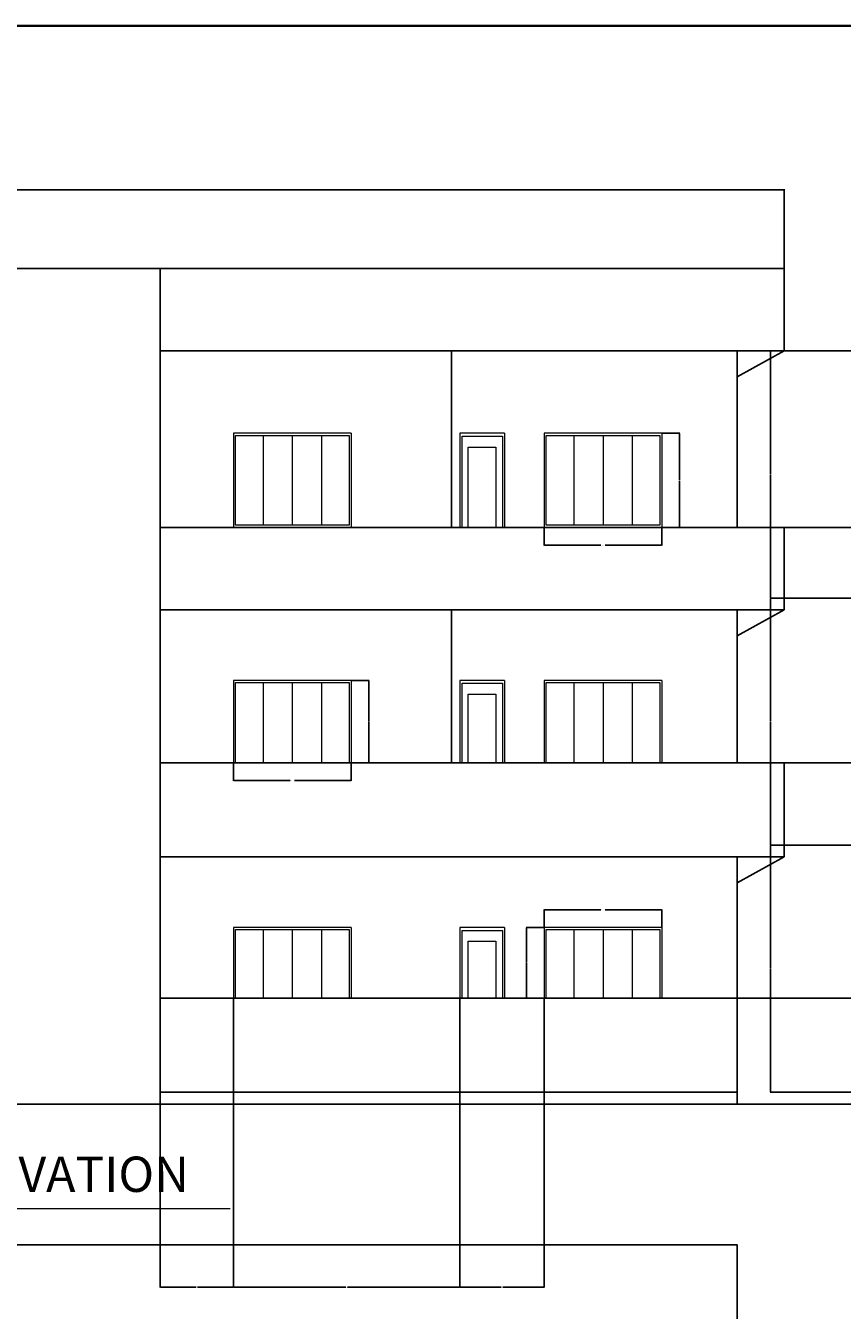
# Model space of a CAD drawing. Units: inches. Extents: x 2120 to 4013, y 1390 to 3019.
# Tile 49 of 59: x 2647 to 3063, y 2364 to 3019. Entities that reach past the tile are written whole.
import ezdxf

# ---------------------------------------------------------------- set-up
doc = ezdxf.new("R2010")
doc.units = ezdxf.units.IN
for name, color, linetype, lineweight in [('A-ANNO-DIMS', 2, 'Continuous', 18), ('A-ANNO-TEXT', 7, 'Continuous', 18), ('A-ANNO-TTLB', 7, 'Continuous', 35), ('A-DOOR', 3, 'Continuous', 18), ('A-ELEV', 7, 'Continuous', 25), ('A-GLAZ', 4, 'Continuous', 18)]:
    doc.layers.add(name, color=color, linetype=linetype, lineweight=lineweight)
doc.styles.get("Standard").update_dxf_attribs({"font": 'arial.ttf'})
doc.dimstyles.get("Standard").update_dxf_attribs({"dimtxt": 0.18, "dimasz": 0.18, "dimexe": 0.18, "dimexo": 0.0625, "dimgap": 0.09, "dimtad": 0, "dimtih": 1, "dimtoh": 1, "dimdec": 4, "dimzin": 0, "dimdsep": 46, "dimtxsty": 'Standard', "dimcen": 0.09, "dimadec": 0, "dimazin": 0, "dimtfac": 1, "dimtdec": 4, "dimtofl": 0, "dimtmove": 0, "dimatfit": 3, "dimfxl": 1, "dimtolj": 1, "dimtzin": 0, "dimarcsym": 0})

# ---------------------------------------------------------------- blocks, each defined once
blk = doc.blocks.new('WIN-ELEV-60IN')
for p, q in [((0, 36), (0, 0)), ((60, 36), (0, 36)), ((0, 36), (0, 0)), ((60, 36), (0, 36)), ((15.15, 34.91), (15.15, 0)), ((30.01, 34.91), (30.01, 0)), ((44.87, 34.91), (44.87, 0)), ((60, 36), (60, 0)), ((60, 36), (60, 0))]:
    blk.add_line(p, q)
blk.add_lwpolyline([(1, 0), (1, 34.91), (59.02, 34.91), (59.02, 0)])
blk = doc.blocks.new('WIN-ELEV-60IN-02')
for p, q in [((0, 42), (0, 0)), ((60, 42), (0, 42)), ((0, 42), (0, 0)), ((60, 42), (0, 42)), ((0, 42), (0, 0)), ((60, 42), (0, 42)), ((15.15, 40.91), (15.15, 0)), ((30.01, 40.91), (30.01, 0)), ((44.87, 40.91), (44.87, 0)), ((60, 42), (60, 0)), ((60, 42), (60, 0)), ((60, 42), (60, 0)), ((0, 36), (0, 0)), ((60, 36), (60, 0))]:
    blk.add_line(p, q)
blk.add_lwpolyline([(1, 0), (1, 40.91), (59.02, 40.91), (59.02, 0)])
blk = doc.blocks.new('WIN-ELEV-60IN-03')
for p, q in [((0, 48), (0, 0)), ((60, 48), (0, 48)), ((0, 48), (0, 0)), ((60, 48), (0, 48)), ((0, 48), (0, 0)), ((60, 48), (0, 48)), ((15.15, 46.91), (15.15, 1.19)), ((30.01, 46.91), (30.01, 1.19)), ((44.87, 46.91), (44.87, 1.19)), ((60, 48), (60, 0)), ((60, 48), (60, 0)), ((60, 48), (60, 0)), ((60, 0), (0, 0)), ((60, 0), (0, 0)), ((60, 0), (0, 0))]:
    blk.add_line(p, q)
blk.add_lwpolyline([(1, 46.91), (59.02, 46.91), (59.02, 1.19), (1, 1.19)], close=True)
blk = doc.blocks.new('*D205')
at = {"layer": 'A-ANNO-DIMS', "color": 0, "lineweight": -2, "transparency": 16777216}
for p, q in [((2911.39, 2559.37), (2911.39, 2568.49)), ((2911.57, 2568.31), (2940.27, 2568.31)), ((2971.21, 2568.31), (2942.51, 2568.31)), ((2971.39, 2559.37), (2971.39, 2568.49))]:
    blk.add_line(p, q, dxfattribs=at)
at = {"layer": 'A-ANNO-DIMS', "color": 0, "transparency": 16777216}
for points in [[(2911.57, 2568.34), (2911.57, 2568.28), (2911.39, 2568.31)], [(2971.21, 2568.34), (2971.21, 2568.28), (2971.39, 2568.31)]]:
    blk.add_solid(points, dxfattribs=at)
at = {"layer": 'Defpoints', "color": 0, "transparency": 16777216}
for p in [(2971.39, 2568.31), (2911.39, 2559.31), (2971.39, 2559.31)]:
    blk.add_point(p, dxfattribs=at)
at = {"layer": 'A-ANNO-DIMS', "color": 0, "transparency": 16777216, "insert": (2941.39, 2568.31), "char_height": 0.18, "attachment_point": 5}
blk.add_mtext('\\A1;WINDOW 60 TYP.', dxfattribs=at)
blk = doc.blocks.new('*D206')
at = {"layer": 'A-ANNO-DIMS', "color": 0, "lineweight": -2, "transparency": 16777216}
for p, q in [((2911.33, 2559.31), (2902.21, 2559.31)), ((2902.39, 2559.13), (2902.39, 2541.49)), ((2902.39, 2523.49), (2902.39, 2541.13)), ((2911.33, 2523.31), (2902.21, 2523.31))]:
    blk.add_line(p, q, dxfattribs=at)
at = {"layer": 'A-ANNO-DIMS', "color": 0, "transparency": 16777216}
for points in [[(2902.36, 2559.13), (2902.42, 2559.13), (2902.39, 2559.31)], [(2902.36, 2523.49), (2902.42, 2523.49), (2902.39, 2523.31)]]:
    blk.add_solid(points, dxfattribs=at)
at = {"layer": 'Defpoints', "color": 0, "transparency": 16777216}
for p in [(2902.39, 2559.31), (2911.39, 2559.31), (2911.39, 2523.31)]:
    blk.add_point(p, dxfattribs=at)
at = {"layer": 'A-ANNO-DIMS', "color": 0, "transparency": 16777216, "insert": (2902.39, 2541.31), "char_height": 0.18, "attachment_point": 5}
blk.add_mtext('\\A1;36 TYP.', dxfattribs=at)
blk = doc.blocks.new('*D207')
at = {"layer": 'A-ANNO-DIMS', "color": 0, "lineweight": -2, "transparency": 16777216}
for p, q in [((2753.02, 2643.25), (2753.02, 2634.13)), ((2813.02, 2643.25), (2813.02, 2634.13)), ((2753.2, 2634.31), (2781.9, 2634.31)), ((2812.84, 2634.31), (2784.14, 2634.31))]:
    blk.add_line(p, q, dxfattribs=at)
at = {"layer": 'A-ANNO-DIMS', "color": 0, "transparency": 16777216}
for points in [[(2753.2, 2634.34), (2753.2, 2634.28), (2753.02, 2634.31)], [(2812.84, 2634.34), (2812.84, 2634.28), (2813.02, 2634.31)]]:
    blk.add_solid(points, dxfattribs=at)
at = {"layer": 'Defpoints', "color": 0, "transparency": 16777216}
for p in [(2753.02, 2643.31), (2813.02, 2643.31), (2813.02, 2634.31)]:
    blk.add_point(p, dxfattribs=at)
at = {"layer": 'A-ANNO-DIMS', "color": 0, "transparency": 16777216, "insert": (2783.02, 2634.31), "char_height": 0.18, "attachment_point": 5}
blk.add_mtext('\\A1;WINDOW 60 TYP.', dxfattribs=at)
blk = doc.blocks.new('*D208')
at = {"layer": 'A-ANNO-DIMS', "color": 0, "lineweight": -2, "transparency": 16777216}
for p, q in [((2813.08, 2685.31), (2822.2, 2685.31)), ((2822.02, 2685.13), (2822.02, 2664.49)), ((2822.02, 2643.49), (2822.02, 2664.13)), ((2813.08, 2643.31), (2822.2, 2643.31))]:
    blk.add_line(p, q, dxfattribs=at)
at = {"layer": 'A-ANNO-DIMS', "color": 0, "transparency": 16777216}
for points in [[(2821.99, 2685.13), (2822.05, 2685.13), (2822.02, 2685.31)], [(2821.99, 2643.49), (2822.05, 2643.49), (2822.02, 2643.31)]]:
    blk.add_solid(points, dxfattribs=at)
at = {"layer": 'Defpoints', "color": 0, "transparency": 16777216}
for p in [(2813.02, 2685.31), (2822.02, 2685.31), (2813.02, 2643.31)]:
    blk.add_point(p, dxfattribs=at)
at = {"layer": 'A-ANNO-DIMS', "color": 0, "transparency": 16777216, "insert": (2822.02, 2664.31), "char_height": 0.18, "attachment_point": 5}
blk.add_mtext('\\A1;42 TYP.', dxfattribs=at)
blk = doc.blocks.new('*D209')
at = {"layer": 'A-ANNO-DIMS', "color": 0, "lineweight": -2, "transparency": 16777216}
for p, q in [((2911.39, 2763.25), (2911.39, 2754.13)), ((2971.39, 2763.25), (2971.39, 2754.13)), ((2911.57, 2754.31), (2940.27, 2754.31)), ((2971.21, 2754.31), (2942.51, 2754.31))]:
    blk.add_line(p, q, dxfattribs=at)
at = {"layer": 'A-ANNO-DIMS', "color": 0, "transparency": 16777216}
for points in [[(2911.57, 2754.34), (2911.57, 2754.28), (2911.39, 2754.31)], [(2971.21, 2754.34), (2971.21, 2754.28), (2971.39, 2754.31)]]:
    blk.add_solid(points, dxfattribs=at)
at = {"layer": 'Defpoints', "color": 0, "transparency": 16777216}
for p in [(2911.39, 2763.31), (2971.39, 2763.31), (2971.39, 2754.31)]:
    blk.add_point(p, dxfattribs=at)
at = {"layer": 'A-ANNO-DIMS', "color": 0, "transparency": 16777216, "insert": (2941.39, 2754.31), "char_height": 0.18, "attachment_point": 5}
blk.add_mtext('\\A1;WINDOW 60 TYP.', dxfattribs=at)
blk = doc.blocks.new('*D210')
at = {"layer": 'A-ANNO-DIMS', "color": 0, "lineweight": -2, "transparency": 16777216}
for p, q in [((2971.45, 2811.31), (2980.57, 2811.31)), ((2980.39, 2811.13), (2980.39, 2787.49)), ((2980.39, 2763.49), (2980.39, 2787.13)), ((2971.45, 2763.31), (2980.57, 2763.31))]:
    blk.add_line(p, q, dxfattribs=at)
at = {"layer": 'A-ANNO-DIMS', "color": 0, "transparency": 16777216}
for points in [[(2980.36, 2811.13), (2980.42, 2811.13), (2980.39, 2811.31)], [(2980.36, 2763.49), (2980.42, 2763.49), (2980.39, 2763.31)]]:
    blk.add_solid(points, dxfattribs=at)
at = {"layer": 'Defpoints', "color": 0, "transparency": 16777216}
for p in [(2971.39, 2811.31), (2980.39, 2811.31), (2971.39, 2763.31)]:
    blk.add_point(p, dxfattribs=at)
at = {"layer": 'A-ANNO-DIMS', "color": 0, "transparency": 16777216, "insert": (2980.39, 2787.31), "char_height": 0.18, "attachment_point": 5}
blk.add_mtext('\\A1;48 TYP.', dxfattribs=at)
blk = doc.blocks.new('*D211')
at = {"layer": 'A-ANNO-DIMS', "color": 0, "lineweight": -2, "transparency": 16777216}
for p, q in [((2262.73, 2352.59), (2262.73, 2397.71)), ((2262.91, 2397.53), (2635.95, 2397.53)), ((3009.55, 2397.53), (2636.52, 2397.53)), ((3009.73, 2352.59), (3009.73, 2397.71))]:
    blk.add_line(p, q, dxfattribs=at)
at = {"layer": 'A-ANNO-DIMS', "color": 0, "transparency": 16777216}
for points in [[(2262.91, 2397.56), (2262.91, 2397.5), (2262.73, 2397.53)], [(3009.55, 2397.56), (3009.55, 2397.5), (3009.73, 2397.53)]]:
    blk.add_solid(points, dxfattribs=at)
at = {"layer": 'Defpoints', "color": 0, "transparency": 16777216}
for p in [(3009.73, 2397.53), (2262.73, 2352.53), (3009.73, 2352.53)]:
    blk.add_point(p, dxfattribs=at)
at = {"layer": 'A-ANNO-DIMS', "color": 0, "transparency": 16777216, "insert": (2636.23, 2397.53), "char_height": 0.18, "attachment_point": 5}
blk.add_mtext('\\A1;747', dxfattribs=at)
blk = doc.blocks.new('*D223')
at = {"layer": 'A-ANNO-DIMS', "color": 0, "lineweight": -2, "transparency": 16777216}
for p, q in [((2238.73, 2895.37), (2238.73, 2935.69)), ((2238.91, 2935.51), (2635.94, 2935.51)), ((3033.55, 2935.51), (2636.52, 2935.51)), ((3033.73, 2895.37), (3033.73, 2935.69))]:
    blk.add_line(p, q, dxfattribs=at)
at = {"layer": 'A-ANNO-DIMS', "color": 0, "transparency": 16777216}
for points in [[(2238.91, 2935.54), (2238.91, 2935.48), (2238.73, 2935.51)], [(3033.55, 2935.54), (3033.55, 2935.48), (3033.73, 2935.51)]]:
    blk.add_solid(points, dxfattribs=at)
at = {"layer": 'Defpoints', "color": 0, "transparency": 16777216}
for p in [(3033.73, 2935.51), (2238.73, 2895.31), (3033.73, 2895.31)]:
    blk.add_point(p, dxfattribs=at)
at = {"layer": 'A-ANNO-DIMS', "color": 0, "transparency": 16777216, "insert": (2636.23, 2935.51), "char_height": 0.18, "attachment_point": 5}
blk.add_mtext('\\A1;795', dxfattribs=at)
blk = doc.blocks.new('*D230')
at = {"layer": 'A-ANNO-DIMS', "color": 0, "lineweight": -2, "transparency": 16777216}
for p, q in [((2715.73, 2523.25), (2715.73, 2375.74)), ((2753.02, 2523.25), (2753.02, 2375.74)), ((2715.91, 2375.92), (2733.98, 2375.92)), ((2752.84, 2375.92), (2734.77, 2375.92))]:
    blk.add_line(p, q, dxfattribs=at)
at = {"layer": 'A-ANNO-DIMS', "color": 0, "transparency": 16777216}
for points in [[(2715.91, 2375.95), (2715.91, 2375.89), (2715.73, 2375.92)], [(2752.84, 2375.95), (2752.84, 2375.89), (2753.02, 2375.92)]]:
    blk.add_solid(points, dxfattribs=at)
at = {"layer": 'Defpoints', "color": 0, "transparency": 16777216}
for p in [(2715.73, 2523.31), (2753.02, 2523.31), (2753.02, 2375.92)]:
    blk.add_point(p, dxfattribs=at)
at = {"layer": 'A-ANNO-DIMS', "color": 0, "transparency": 16777216, "insert": (2734.38, 2375.92), "char_height": 0.18, "attachment_point": 5}
blk.add_mtext('\\A1;37.29', dxfattribs=at)
blk = doc.blocks.new('*D231')
at = {"layer": 'A-ANNO-DIMS', "color": 0, "lineweight": -2, "transparency": 16777216}
for p, q in [((2753.02, 2523.25), (2753.02, 2375.74)), ((2868.41, 2523.25), (2868.41, 2375.74)), ((2753.2, 2375.92), (2810.33, 2375.92)), ((2868.23, 2375.92), (2811.1, 2375.92))]:
    blk.add_line(p, q, dxfattribs=at)
at = {"layer": 'A-ANNO-DIMS', "color": 0, "transparency": 16777216}
for points in [[(2753.2, 2375.95), (2753.2, 2375.89), (2753.02, 2375.92)], [(2868.23, 2375.95), (2868.23, 2375.89), (2868.41, 2375.92)]]:
    blk.add_solid(points, dxfattribs=at)
at = {"layer": 'Defpoints', "color": 0, "transparency": 16777216}
for p in [(2753.02, 2523.31), (2868.41, 2523.31), (2868.41, 2375.92)]:
    blk.add_point(p, dxfattribs=at)
at = {"layer": 'A-ANNO-DIMS', "color": 0, "transparency": 16777216, "insert": (2810.72, 2375.92), "char_height": 0.18, "attachment_point": 5}
blk.add_mtext('\\A1;115.4', dxfattribs=at)
blk = doc.blocks.new('*D232')
at = {"layer": 'A-ANNO-DIMS', "color": 0, "lineweight": -2, "transparency": 16777216}
for p, q in [((2868.41, 2523.25), (2868.41, 2375.74)), ((2911.39, 2523.25), (2911.39, 2375.74)), ((2868.59, 2375.92), (2889.5, 2375.92)), ((2911.21, 2375.92), (2890.3, 2375.92))]:
    blk.add_line(p, q, dxfattribs=at)
at = {"layer": 'A-ANNO-DIMS', "color": 0, "transparency": 16777216}
for points in [[(2868.59, 2375.95), (2868.59, 2375.89), (2868.41, 2375.92)], [(2911.21, 2375.95), (2911.21, 2375.89), (2911.39, 2375.92)]]:
    blk.add_solid(points, dxfattribs=at)
at = {"layer": 'Defpoints', "color": 0, "transparency": 16777216}
for p in [(2868.41, 2523.31), (2911.39, 2523.31), (2911.39, 2375.92)]:
    blk.add_point(p, dxfattribs=at)
at = {"layer": 'A-ANNO-DIMS', "color": 0, "transparency": 16777216, "insert": (2889.9, 2375.92), "char_height": 0.18, "attachment_point": 5}
blk.add_mtext('\\A1;42.98', dxfattribs=at)
blk = doc.blocks.new('*D233')
at = {"layer": 'A-ANNO-DIMS', "color": 0, "lineweight": -2, "transparency": 16777216}
for p, q in [((3009.8, 2523.31), (3074.11, 2523.31)), ((3073.93, 2523.13), (3073.93, 2496.49)), ((3073.93, 2469.49), (3073.93, 2496.13)), ((3009.8, 2469.31), (3074.11, 2469.31))]:
    blk.add_line(p, q, dxfattribs=at)
at = {"layer": 'A-ANNO-DIMS', "color": 0, "transparency": 16777216}
for points in [[(3073.9, 2523.13), (3073.96, 2523.13), (3073.93, 2523.31)], [(3073.9, 2469.49), (3073.96, 2469.49), (3073.93, 2469.31)]]:
    blk.add_solid(points, dxfattribs=at)
at = {"layer": 'Defpoints', "color": 0, "transparency": 16777216}
for p in [(3009.73, 2523.31), (3073.93, 2523.31), (3009.73, 2469.31)]:
    blk.add_point(p, dxfattribs=at)
at = {"layer": 'A-ANNO-DIMS', "color": 0, "transparency": 16777216, "insert": (3073.93, 2496.31), "char_height": 0.18, "attachment_point": 5}
blk.add_mtext('\\A1;54', dxfattribs=at)
blk = doc.blocks.new('*D234')
at = {"layer": 'A-ANNO-DIMS', "color": 0, "lineweight": -2, "transparency": 16777216}
for p, q in [((3033.8, 2643.31), (3074.11, 2643.31)), ((3073.93, 2643.13), (3073.93, 2583.49)), ((3073.93, 2523.49), (3073.93, 2583.13)), ((3009.8, 2523.31), (3074.11, 2523.31))]:
    blk.add_line(p, q, dxfattribs=at)
at = {"layer": 'A-ANNO-DIMS', "color": 0, "transparency": 16777216}
for points in [[(3073.9, 2643.13), (3073.96, 2643.13), (3073.93, 2643.31)], [(3073.9, 2523.49), (3073.96, 2523.49), (3073.93, 2523.31)]]:
    blk.add_solid(points, dxfattribs=at)
at = {"layer": 'Defpoints', "color": 0, "transparency": 16777216}
for p in [(3033.73, 2643.31), (3073.93, 2643.31), (3009.73, 2523.31)]:
    blk.add_point(p, dxfattribs=at)
at = {"layer": 'A-ANNO-DIMS', "color": 0, "transparency": 16777216, "insert": (3073.93, 2583.31), "char_height": 0.18, "attachment_point": 5}
blk.add_mtext('\\A1;120', dxfattribs=at)
blk = doc.blocks.new('*D235')
at = {"layer": 'A-ANNO-DIMS', "color": 0, "lineweight": -2, "transparency": 16777216}
for p, q in [((3033.8, 2763.31), (3074.11, 2763.31)), ((3073.93, 2763.13), (3073.93, 2703.49)), ((3073.93, 2643.49), (3073.93, 2703.13)), ((3033.8, 2643.31), (3074.11, 2643.31))]:
    blk.add_line(p, q, dxfattribs=at)
at = {"layer": 'A-ANNO-DIMS', "color": 0, "transparency": 16777216}
for points in [[(3073.9, 2763.13), (3073.96, 2763.13), (3073.93, 2763.31)], [(3073.9, 2643.49), (3073.96, 2643.49), (3073.93, 2643.31)]]:
    blk.add_solid(points, dxfattribs=at)
at = {"layer": 'Defpoints', "color": 0, "transparency": 16777216}
for p in [(3033.73, 2763.31), (3073.93, 2763.31), (3033.73, 2643.31)]:
    blk.add_point(p, dxfattribs=at)
at = {"layer": 'A-ANNO-DIMS', "color": 0, "transparency": 16777216, "insert": (3073.93, 2703.31), "char_height": 0.18, "attachment_point": 5}
blk.add_mtext('\\A1;120', dxfattribs=at)
blk = doc.blocks.new('*D238')
at = {"layer": 'A-ANNO-DIMS', "color": 0, "lineweight": -2, "transparency": 16777216}
for p, q in [((3071.67, 2601.31), (3026.6, 2601.31)), ((3026.78, 2601.13), (3026.78, 2538.49)), ((3026.78, 2475.49), (3026.78, 2538.13)), ((3071.67, 2475.31), (3026.6, 2475.31))]:
    blk.add_line(p, q, dxfattribs=at)
at = {"layer": 'A-ANNO-DIMS', "color": 0, "transparency": 16777216}
for points in [[(3026.75, 2601.13), (3026.81, 2601.13), (3026.78, 2601.31)], [(3026.75, 2475.49), (3026.81, 2475.49), (3026.78, 2475.31)]]:
    blk.add_solid(points, dxfattribs=at)
at = {"layer": 'Defpoints', "color": 0, "transparency": 16777216}
for p in [(3026.78, 2601.31), (3071.73, 2601.31), (3071.73, 2475.31)]:
    blk.add_point(p, dxfattribs=at)
at = {"layer": 'A-ANNO-DIMS', "color": 0, "transparency": 16777216, "insert": (3026.78, 2538.31), "char_height": 0.18, "attachment_point": 5}
blk.add_mtext('\\A1;126', dxfattribs=at)
blk = doc.blocks.new('*D239')
at = {"layer": 'A-ANNO-DIMS', "color": 0, "lineweight": -2, "transparency": 16777216}
for p, q in [((3071.67, 2727.31), (3026.6, 2727.31)), ((3026.78, 2727.13), (3026.78, 2664.49)), ((3026.78, 2601.49), (3026.78, 2664.13)), ((3071.67, 2601.31), (3026.6, 2601.31))]:
    blk.add_line(p, q, dxfattribs=at)
at = {"layer": 'A-ANNO-DIMS', "color": 0, "transparency": 16777216}
for points in [[(3026.75, 2727.13), (3026.81, 2727.13), (3026.78, 2727.31)], [(3026.75, 2601.49), (3026.81, 2601.49), (3026.78, 2601.31)]]:
    blk.add_solid(points, dxfattribs=at)
at = {"layer": 'Defpoints', "color": 0, "transparency": 16777216}
for p in [(3026.78, 2727.31), (3071.73, 2727.31), (3071.73, 2601.31)]:
    blk.add_point(p, dxfattribs=at)
at = {"layer": 'A-ANNO-DIMS', "color": 0, "transparency": 16777216, "insert": (3026.78, 2664.31), "char_height": 0.18, "attachment_point": 5}
blk.add_mtext('\\A1;126', dxfattribs=at)
blk = doc.blocks.new('*D240')
at = {"layer": 'A-ANNO-DIMS', "color": 0, "lineweight": -2, "transparency": 16777216}
for p, q in [((3071.67, 2853.31), (3026.6, 2853.31)), ((3026.78, 2853.13), (3026.78, 2790.49)), ((3026.78, 2727.49), (3026.78, 2790.13)), ((3071.67, 2727.31), (3026.6, 2727.31))]:
    blk.add_line(p, q, dxfattribs=at)
at = {"layer": 'A-ANNO-DIMS', "color": 0, "transparency": 16777216}
for points in [[(3026.75, 2853.13), (3026.81, 2853.13), (3026.78, 2853.31)], [(3026.75, 2727.49), (3026.81, 2727.49), (3026.78, 2727.31)]]:
    blk.add_solid(points, dxfattribs=at)
at = {"layer": 'Defpoints', "color": 0, "transparency": 16777216}
for p in [(3026.78, 2853.31), (3071.73, 2853.31), (3071.73, 2727.31)]:
    blk.add_point(p, dxfattribs=at)
at = {"layer": 'A-ANNO-DIMS', "color": 0, "transparency": 16777216, "insert": (3026.78, 2790.31), "char_height": 0.18, "attachment_point": 5}
blk.add_mtext('\\A1;126', dxfattribs=at)

msp = doc.modelspace()

# ---------------------------------------------------------------- linework, layer by layer
at = {"layer": 'A-ANNO-TEXT'}
msp.add_line((2586.5728, 2416.1241), (2751.3079, 2416.1241), dxfattribs=at)
at = {"layer": 'A-ANNO-TTLB'}
msp.add_lwpolyline([(2120.4581, 3019.1237), (4012.9334, 3019.1237), (4012.9334, 1390.2222), (2120.4581, 1390.2222)], close=True, dxfattribs=at)
at = {"layer": 'A-DOOR'}
for p, q in [((2868.4123, 2811.3118), (2868.4123, 2763.3118)), ((2891.2137, 2811.3118), (2868.4123, 2811.3118)), ((2868.4123, 2811.3118), (2868.4123, 2763.3118)), ((2891.2137, 2811.3118), (2868.4123, 2811.3118)), ((2891.2137, 2811.3118), (2891.2137, 2763.3118)), ((2891.2137, 2811.3118), (2891.2137, 2763.3118)), ((2868.4123, 2685.3118), (2868.4123, 2643.3118)), ((2891.2137, 2685.3118), (2868.4123, 2685.3118)), ((2868.4123, 2685.3118), (2868.4123, 2643.3118)), ((2891.2137, 2685.3118), (2868.4123, 2685.3118)), ((2868.4123, 2679.3118), (2868.4123, 2643.3118)), ((2891.2137, 2685.3118), (2891.2137, 2643.3118)), ((2891.2137, 2685.3118), (2891.2137, 2643.3118)), ((2891.2137, 2679.3118), (2891.2137, 2643.3118)), ((2868.4123, 2559.3118), (2868.4123, 2523.3118)), ((2891.2137, 2559.3118), (2868.4123, 2559.3118)), ((2891.2137, 2559.3118), (2891.2137, 2523.3118))]:
    msp.add_line(p, q, dxfattribs=at)
for points in [[(2869.5464, 2763.3118), (2869.5464, 2809.8247), (2890.209, 2809.8247), (2890.209, 2763.3118)], [(2872.722, 2763.3118), (2872.722, 2804.2987), (2886.8441, 2804.2987), (2886.8441, 2763.3118)], [(2869.5464, 2643.3118), (2869.5464, 2683.8247), (2890.209, 2683.8247), (2890.209, 2643.3118)], [(2872.722, 2643.3118), (2872.722, 2678.2987), (2886.8441, 2678.2987), (2886.8441, 2643.3118)], [(2869.5464, 2523.3118), (2869.5464, 2557.8247), (2890.209, 2557.8247), (2890.209, 2523.3118)], [(2872.722, 2523.3118), (2872.722, 2552.2987), (2886.8441, 2552.2987), (2886.8441, 2523.3118)]]:
    msp.add_lwpolyline(points, dxfattribs=at)
at = {"layer": 'A-ELEV'}
for p, q in [((2637.7331, 2895.3118), (2715.7331, 2895.3118)), ((2715.7331, 2895.3118), (2715.7331, 2727.3118)), ((3033.7331, 2895.3118), (2715.7331, 2895.3118)), ((3033.7331, 2853.3118), (3033.7331, 2895.3118)), ((3033.7331, 2853.3118), (2715.7331, 2853.3118)), ((2864.2331, 2853.3118), (2864.2331, 2763.3118)), ((3009.7331, 2853.3118), (3009.7331, 2763.3118)), ((3009.7331, 2853.3118), (3009.7331, 2763.3118)), ((3033.7331, 2853.3118), (3009.7331, 2840.0471)), ((3033.7331, 2853.3118), (3033.7331, 2853.3118)), ((3009.7331, 2840.0471), (3009.7331, 2840.0471)), ((3009.7331, 2769.3118), (3009.7331, 2763.3118)), ((3033.7331, 2763.3118), (2715.7331, 2763.3118)), ((2715.7331, 2763.3118), (2715.7331, 2601.3118)), ((3033.7331, 2721.3118), (3033.7331, 2763.3118)), ((2715.7331, 2721.3118), (2715.7331, 2595.3118)), ((3033.7331, 2721.3118), (2715.7331, 2721.3118)), ((2864.2331, 2721.3118), (2864.2331, 2643.3118)), ((3009.7331, 2721.3118), (3009.7331, 2643.3118)), ((3033.7331, 2721.3118), (3009.7331, 2708.0471)), ((3009.7331, 2721.3118), (3009.7331, 2643.3118)), ((3009.7331, 2721.3118), (3009.7331, 2709.3118)), ((3009.7331, 2721.3118), (3009.7331, 2643.3118)), ((2715.7331, 2643.3118), (2715.7331, 2469.3118)), ((3033.7331, 2643.3118), (2715.7331, 2643.3118)), ((3033.7331, 2595.3118), (3033.7331, 2643.3118)), ((3033.7331, 2595.3118), (2715.7331, 2595.3118)), ((3033.7331, 2595.3118), (3009.7331, 2582.0471)), ((3009.7331, 2523.3118), (3009.7331, 2595.3118)), ((3009.7331, 2595.3118), (3009.7331, 2469.3118)), ((2715.7331, 2523.3118), (3009.7331, 2523.3118)), ((2637.7331, 2469.3118), (2715.7331, 2469.3118)), ((3009.7331, 2475.3118), (2715.7331, 2475.3118)), ((2715.7331, 2469.3118), (3009.7331, 2469.3118)), ((2715.7331, 2469.3118), (2715.7331, 2469.3118))]:
    msp.add_line(p, q, dxfattribs=at)

# ---------------------------------------------------------------- block references
at = {"layer": 'A-GLAZ'}
for name, p in [('WIN-ELEV-60IN-03', (2753.02, 2763.3118)), ('WIN-ELEV-60IN-02', (2753.02, 2643.3118)), ('WIN-ELEV-60IN', (2753.02, 2523.3118))]:
    msp.add_blockref(name, p, dxfattribs=at)
for name, p, rotation in [('WIN-ELEV-60IN-03', (2911.3921, 2763.3118), 359.9999776546053), ('WIN-ELEV-60IN-02', (2911.3921, 2643.3118), 7.4430260893e-06), ('WIN-ELEV-60IN', (2911.3921, 2523.3118), 3.8181918208e-06)]:
    msp.add_blockref(name, p, dxfattribs=dict(at, rotation=rotation))

# ---------------------------------------------------------------- texts
at = {"layer": 'A-ANNO-TEXT', "insert": (2601.1859, 2442.5081), "char_height": 18, "attachment_point": 1}
msp.add_mtext_dynamic_manual_height_columns('ELEVATION', width=359.82979, gutter_width=12.5, heights=[0], dxfattribs=at)

# ---------------------------------------------------------------- dimensions: what is measured, and where the dimension line sits
at = {"layer": 'A-ANNO-DIMS'}
for base, p1, p2, override, picture, middle in [((3033.7331, 2935.5118), (2238.7331, 2895.3118), (3033.7331, 2895.3118), {"dimdec": 0, "dimlfac": 1, "dimrnd": 0, "dimzin": 0, "dimdsep": 46, "dimlunit": 2}, '*D223', (2636.2331, 2935.5118)), ((2753.02, 2375.9241), (2715.7331, 2523.3118), (2753.02, 2523.3118), {"dimdec": 2, "dimlfac": 1, "dimrnd": 0, "dimzin": 0, "dimdsep": 46, "dimlunit": 2}, '*D230', (2734.3766, 2375.9241)), ((2868.4123, 2375.9241), (2753.02, 2523.3118), (2868.4123, 2523.3118), {"dimdec": 1, "dimlfac": 1, "dimrnd": 0, "dimzin": 0, "dimdsep": 46, "dimlunit": 2}, '*D231', (2810.7162, 2375.9241)), ((2911.3921, 2375.9241), (2868.4123, 2523.3118), (2911.3921, 2523.3118), {"dimdec": 2, "dimlfac": 1, "dimrnd": 0, "dimzin": 0, "dimdsep": 46, "dimlunit": 2}, '*D232', (2889.9022, 2375.9241)), ((3009.7331, 2397.531), (2262.7331, 2352.531), (3009.7331, 2352.531), {"dimdec": 0, "dimlfac": 1, "dimrnd": 0, "dimzin": 0, "dimdsep": 46, "dimlunit": 2}, '*D211', (2636.2331, 2397.531))]:
    dim = msp.add_linear_dim(base=base, p1=p1, p2=p2, dimstyle='Standard', override=override, dxfattribs=at)
    dim.commit()
    dim.dimension.update_dxf_attribs({"geometry": picture, "text_midpoint": middle})
for base, p1, p2, picture, middle in [((3026.7847, 2853.3118), (3071.7347, 2727.3118), (3071.7347, 2853.3118), '*D240', (3026.7847, 2790.3118)), ((3073.9331, 2763.3118), (3033.7331, 2643.3118), (3033.7331, 2763.3118), '*D235', (3073.9331, 2703.3118)), ((3026.7847, 2727.3118), (3071.7347, 2601.3118), (3071.7347, 2727.3118), '*D239', (3026.7847, 2664.3118)), ((3073.9331, 2643.3118), (3009.7331, 2523.3118), (3033.7331, 2643.3118), '*D234', (3073.9331, 2583.3118)), ((3026.7847, 2601.3118), (3071.7347, 2475.3118), (3071.7347, 2601.3118), '*D238', (3026.7847, 2538.3118)), ((3073.9331, 2523.3118), (3009.7331, 2469.3118), (3009.7331, 2523.3118), '*D233', (3073.9331, 2496.3118))]:
    dim = msp.add_linear_dim(base=base, p1=p1, p2=p2, angle=90, dimstyle='Standard', override={"dimdec": 0, "dimlfac": 1, "dimrnd": 0, "dimzin": 0, "dimdsep": 46, "dimlunit": 2}, dxfattribs=at)
    dim.commit()
    dim.dimension.update_dxf_attribs({"geometry": picture, "text_midpoint": middle})
for base, p1, p2, angle, text, picture, middle in [((2980.3921, 2811.3118), (2971.3921, 2763.3118), (2971.3921, 2811.3118), 89.9999777, '<> TYP.', '*D210', (2980.3921, 2787.3118)), ((2971.3921, 2754.3118), (2911.3921, 2763.3118), (2971.3921, 2763.3118), 359.9999777, 'WINDOW <> TYP.', '*D209', (2941.3921, 2754.3118)), ((2822.02, 2685.3118), (2813.02, 2643.3118), (2813.02, 2685.3118), 90, '<> TYP.', '*D208', (2822.02, 2664.3118)), ((2971.3921, 2568.3118), (2911.3921, 2559.3118), (2971.3921, 2559.3118), 0.0000038, 'WINDOW <> TYP.', '*D205', (2941.3921, 2568.3118)), ((2902.3921, 2559.3118), (2911.3921, 2523.3118), (2911.3921, 2559.3118), 90.0000038, '<> TYP.', '*D206', (2902.3921, 2541.3118))]:
    dim = msp.add_linear_dim(base=base, p1=p1, p2=p2, angle=angle, text=text, dimstyle='Standard', override={"dimdec": 0, "dimlfac": 1, "dimrnd": 0, "dimzin": 0, "dimdsep": 46, "dimlunit": 2}, dxfattribs=at)
    dim.commit()
    dim.dimension.update_dxf_attribs({"geometry": picture, "text_midpoint": middle})
dim = msp.add_linear_dim(base=(2813.02, 2634.3118), p1=(2753.02, 2643.3118), p2=(2813.02, 2643.3118), text='WINDOW <> TYP.', dimstyle='Standard', override={"dimdec": 0, "dimlfac": 1, "dimrnd": 0, "dimzin": 0, "dimdsep": 46, "dimlunit": 2}, dxfattribs=at)
dim.commit()
dim.dimension.update_dxf_attribs({"geometry": '*D207', "text_midpoint": (2783.02, 2634.3118)})

doc.saveas('drawing.dxf')
